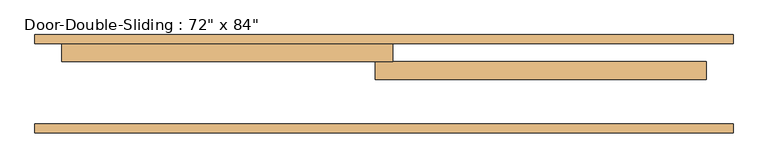
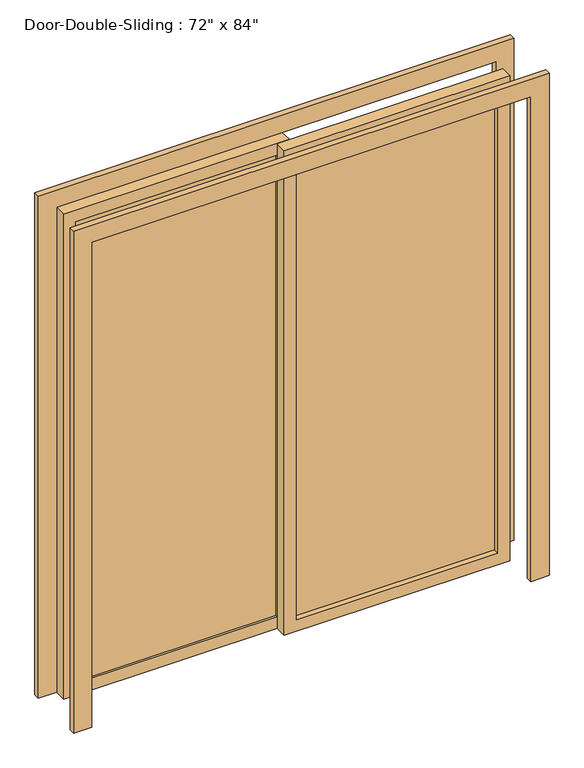
"""IFC4 building model written with IfcOpenShell, lengths in millimetres: door geometry."""

from ifc_helpers import new_model, si_unit, frame, origin, place, context, project, spatial, polyline, outline, extrude, source, transform, mapped, element, save


def door_d4d75d1e(model_context):
    return source(origin(), model_context, "Body", "SweptSolid", [
        extrude(outline(polyline([(0.0, 990.6), (2209.8, 990.6), (2209.8, -990.6), (0.0, -990.6), (0.0, -914.4), (2133.6, -914.4), (2133.6, 914.4), (0.0, 914.4), (0.0, 990.6)])), frame((0.0, 241.3, 0.0), z_axis=(0.0, 1.0, 0.0), x_axis=(0.0, 0.0, 1.0)), (0.0, 0.0, 1.0), 25.4),
        extrude(outline(polyline([(0.0, -990.6), (0.0, -914.4), (2133.6, -914.4), (2133.6, 914.4), (0.0, 914.4), (0.0, 990.6), (2209.8, 990.6), (2209.8, -990.6), (0.0, -990.6)])), frame((0.0, -12.7, 0.0), z_axis=(0.0, 1.0, 0.0), x_axis=(0.0, 0.0, 1.0)), (0.0, 0.0, 1.0), 25.4),
        extrude(outline(polyline([(2133.6, 25.4), (2133.6, -914.4), (0.0, -914.4), (0.0, 25.4), (2133.6, 25.4)]), holes=[polyline([(2082.8, -25.4), (50.8, -25.4), (50.8, -863.6), (2082.8, -863.6), (2082.8, -25.4)])]), frame((0.0, 190.5, 0.0), z_axis=(0.0, 1.0, 0.0), x_axis=(0.0, 0.0, 1.0)), (0.0, 0.0, 1.0), 50.8),
        extrude(outline(polyline([(2133.6, -25.4), (0.0, -25.4), (0.0, 914.4), (2133.6, 914.4), (2133.6, -25.4)]), holes=[polyline([(2082.8, 25.4), (2082.8, 863.6), (50.8, 863.6), (50.8, 25.4), (2082.8, 25.4)])]), frame((0.0, 139.7, 0.0), z_axis=(0.0, 1.0, 0.0), x_axis=(0.0, 0.0, 1.0)), (0.0, 0.0, 1.0), 50.8),
        extrude(outline(polyline([(-25.4, 200.025), (-863.6, 200.025), (-863.6, 206.375), (-25.4, 206.375), (-25.4, 200.025)])), frame((0.0, 0.0, 50.8), z_axis=(0.0, 0.0, 1.0), x_axis=(1.0, 0.0, 0.0)), (0.0, 0.0, 1.0), 2032.0),
        extrude(outline(polyline([(25.4, 168.275), (863.6, 168.275), (863.6, 161.925), (25.4, 161.925), (25.4, 168.275)])), frame((0.0, 0.0, 50.8), z_axis=(0.0, 0.0, 1.0), x_axis=(1.0, 0.0, 0.0)), (0.0, 0.0, 1.0), 2032.0),
    ])


if __name__ == "__main__":
    model = new_model("IFC4")
    model_context = context("Model", 3, world=origin())
    ifc_project = project(units=[si_unit("LENGTHUNIT", "METRE", prefix="MILLI")], contexts=[model_context])
    site = spatial("IfcSite", under=ifc_project)
    building = spatial("IfcBuilding", under=site)
    placement = place(None, origin())
    door_shape = door_d4d75d1e(model_context)
    element("IfcDoor", 1, ObjectType="Door-Double-Sliding : 72\" x 84\"", at=placement, inside=building, context=model_context, shape_type="MappedRepresentation", body=[
        mapped(door_shape, transform((0.0, 0.0, 0.0), x_axis=(1.0, 0.0, 0.0), y_axis=(0.0, 1.0, 0.0), z_axis=(0.0, 0.0, 1.0))),
    ])
    save(model, "model.ifc")

# Revit data of these elements
# Type "Door-Double-Sliding : 72\" x 84\""
#   Type Mark = "11"
#   Construction Type Id = "opn-d45"
#   Assembly Code = "C1020"
#   Analytic Construction = "Wood frame, double glass door "
#   Thickness = 0' - 2"
#   Thermal Resistance (R) = 1.8150 (h·ft²·°F)/BTU
#   Heat Transfer Coefficient (U) = 0.5510 BTU/(h·ft²·°F)
#   Height = 7' - 0"
#   Rail Width = 0' - 2"
#   Stiles = 0' - 2"
#   Trim Projection Ext = 0' - 1"
#   Trim Projection Int = 0' - 1"
#   Trim Width = 0' - 3"
#   Width = 6' - 0"
#   Define Thermal Properties by = 1
#   Glazing = Glass
#   Panel Material = Wood - Birch - Solid Stained Light Low Gloss
#   Trim Material = Paint - Sienna
#   Visual Light Transmittance = 0
#   Solar Heat Gain Coefficient = 0
#   Function = (empty or 0)
#   Wall Closure = (empty or 0)
# Element 1 (IfcDoor, "Door-Double-Sliding : 72\" x 84\"")
#   Materials on its faces: "Paint - Sienna", "Wood - Birch - Solid Stained Light Low Gloss", "Glass"
# Materials
#   "Glass": class "Glass", colour RGB 0 128 192, transparency 0.75, Description = "Soda Lime Glass", Cost = 0
#   "Wood - Birch - Solid Stained Light Low Gloss": class "Wood", colour RGB 210 159 95, transparency 0, Cost = 0
#   "Paint - Sienna": colour RGB 118 70 51, transparency 0, Cost = 0
